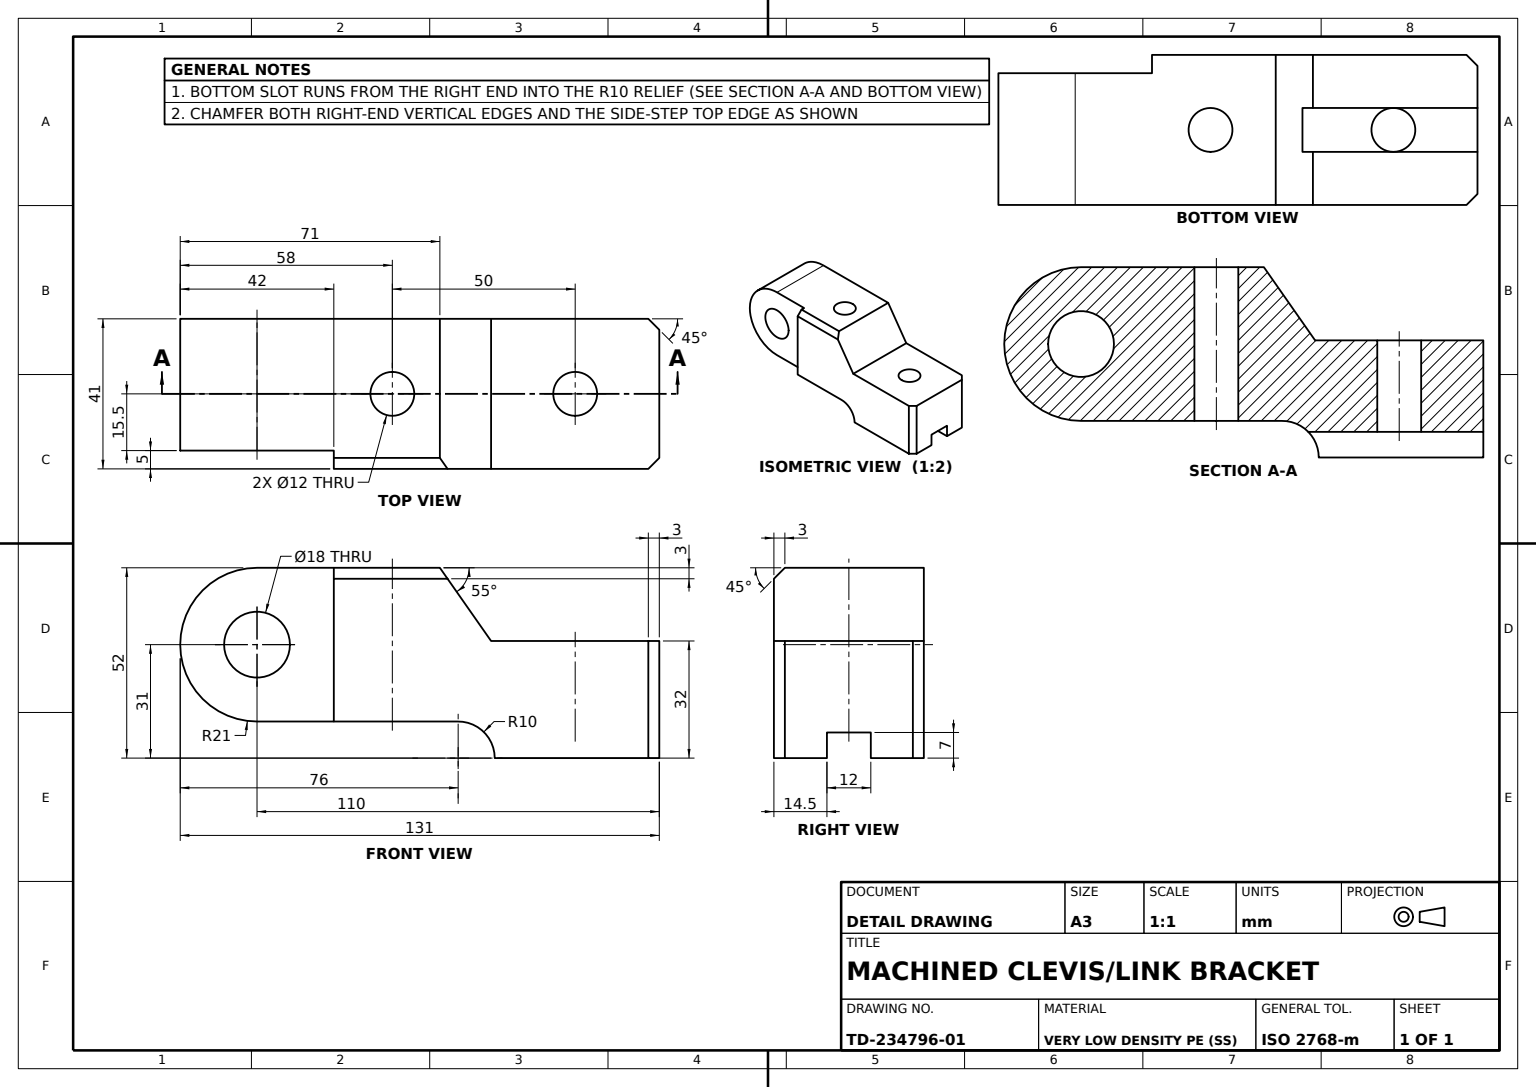
SolidWorks part; units mm, degrees
material "Very Low Density PE (SS)"
ref_plane "Front Plane" through (0, 0, 0) normal (0, 0, 1) x (1, 0, 0)
ref_plane "Top Plane" through (0, 0, 0) normal (0, 1, 0) x (1, 0, 0)
ref_plane "Right Plane" through (0, 0, 0) normal (1, 0, 0) x (0, 0, -1)
sketch "Bracket Side Profile Sketch" plane through (0, 0, 0) normal (0, 0, 1) x (1, 0, 0)
  line L0 (0, 0) -> (-45, 0)
  line L1 (-55.1684, 9.9986) -> (-86.001, 9.9986)
  line L3 (-85.9968, 51.9986) -> (-60, 51.9986)
  line L4 (-60, 51.9986) -> (-45.9968, 32)
  line L5 (-45.9968, 32) -> (0, 32)
  line L6 (0, 32) -> (0, 0)
  line L7 (-110, 51.9986) -> (-85.9968, 51.9986)
  line L8 (-110, 9.9986) -> (-86.001, 9.9986)
  line L10 (-72.9984, 51.9986) -> (-72.9984, 69.578) construction
  line L11 (-22.9984, 32) -> (-22.9984, 73.7407) construction
  arc A0 (-45, 0) -> (-55.1684, 9.9986) centre (-55, 0) ccw
  circle A1 centre (-110, 30.9986) radius 9
  arc A2 (-110, 51.9986) -> (-110, 9.9986) centre (-110, 30.9986) ccw
  dimension "D4" = 10
  dimension "D8" = 18
  dimension "D9" = 42
  dimension "D10" = 22.0014
  dimension "D1" = 45
  dimension "D2" = 32
  dimension "D3" = 55
  dimension "D5" = 110
  dimension "D6" = 42
  dimension "D7" = 50
  dimension "50" = 50
  dimension "D11" = 23.999
extrude "Bracket Body 41mm" add sketch "Bracket Side Profile Sketch" along normal mid plane 41
sketch "Top Face Cuts Sketch" plane through (0, 51.9986, 0) normal (0, 1, 0) x (1, 0, 0)
  line L0 (-22.9984, -20.5) -> (-22.9984, 0) construction
  line L1 (0, -20.5) -> (-45.9968, -20.5) construction
  line L2 (-131, -15.5) -> (-89, -15.5)
  line L3 (-131, 20.5) -> (-131, -20.5) construction
  line L4 (-89, -15.5) -> (-89, -20.5)
  line L5 (-60, -20.5) -> (-110, -20.5) construction
  line L6 (-89, -20.5) -> (-131, -20.5)
  line L7 (-131, -20.5) -> (-131, -15.5)
  line L9 (-60, 20.5) -> (-110, 20.5) construction
  circle A0 centre (-72.9984, 0) radius 6
  circle A1 centre (-22.9984, 0) radius 6
  dimension "D1" = 50
  dimension "D2" = 12
  dimension "D3" = 5
  dimension "D4" = 42
  dimension "D5" = 20.5
extrude "Top Face Cuts" cut sketch "Top Face Cuts Sketch" against normal through all
sketch "End Slot Sketch" plane through (0, 0, 0) normal (1, 0, 0) x (0, 0, -1)
  line L0 (-6, 0) -> (-6, 7)
  line L1 (-20.5, 0) -> (20.5, 0) construction
  line L2 (-6, 7) -> (6, 7)
  line L3 (6, 7) -> (6, 0)
  line L4 (6, 0) -> (-6, 0)
  dimension "D1" = 12
  dimension "D2" = 7
  dimension "D3" = 6
extrude "End Slot 12mm" cut sketch "End Slot Sketch" against normal through all
chamfer "Edge Chamfer 3mm" distance 3 angle 45 3 edges at (0, 16, -20.5) (0, 16, 20.5) (-74.5, 51.9986, 20.5)
